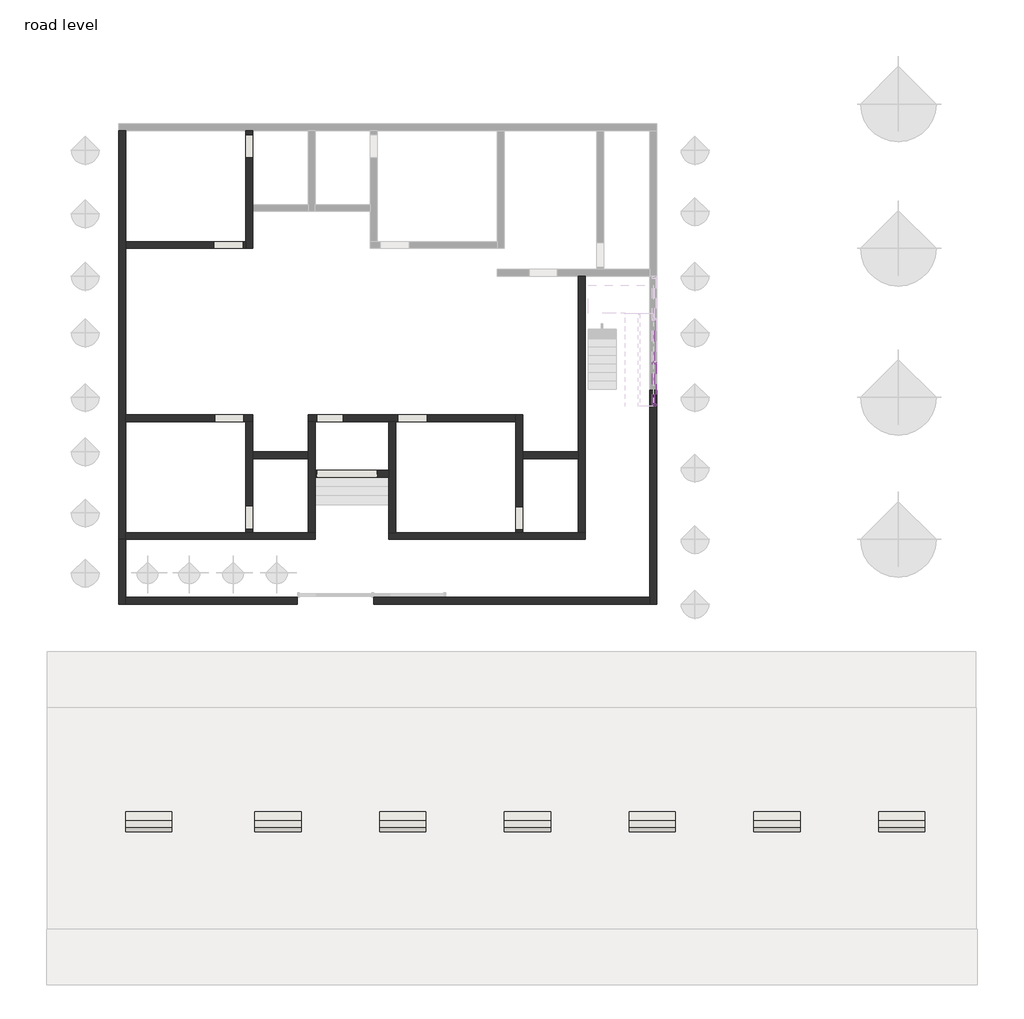
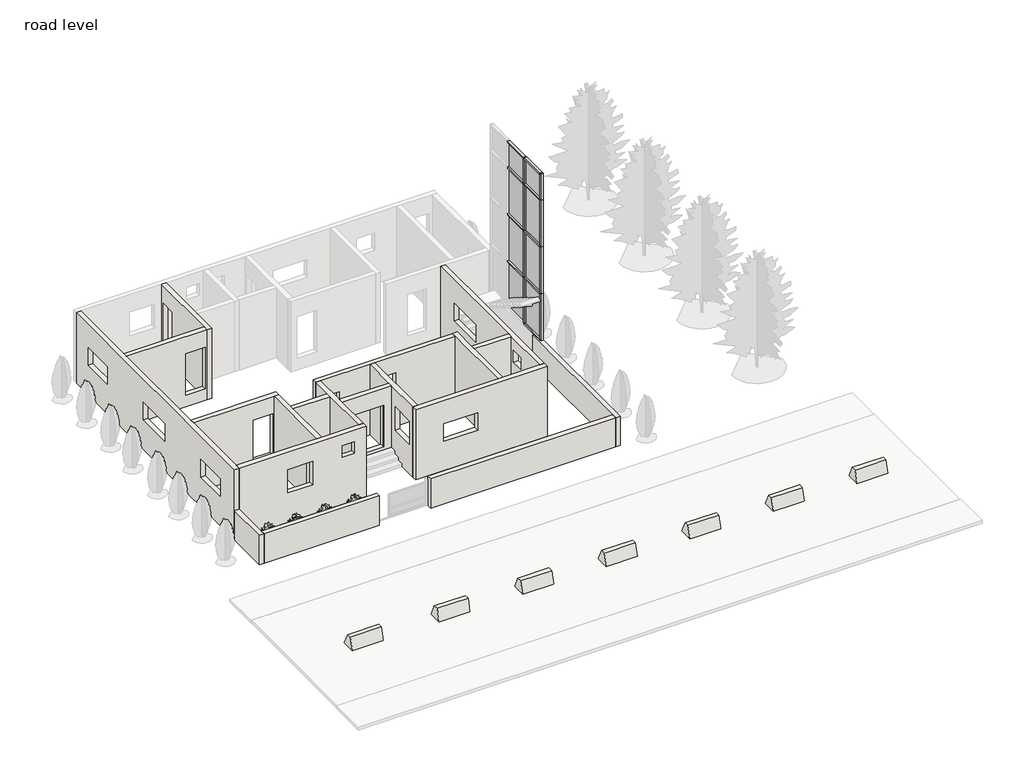
# One storey, part 1 of 2: 26 walls, 17 members, 8 plates.
"""IFC4 building model written with IfcOpenShell, lengths in millimetres."""

from ifc_helpers import new_model, si_unit, frame, origin, origin_with_axes, place, context, project, spatial, polyline, outline, extrude, faceted_brep, transform, mapped, element, save
from components import member_6e705821, member_22948727, member_0bf151aa, member_30211588, member_f0fea5a5, member_ee409385, member_824a4a8d, member_c6627131, system_panel_glazed_532211e4, system_panel_glazed_fddb435e, system_panel_glazed_e2c3efe7, system_panel_glazed_aadce453, system_panel_glazed_7e5d82eb, system_panel_glazed_fa23d52e

model = new_model("IFC4")

# Units and contexts
model_context = context("Model", 3, world=origin())
ifc_project = project(units=[si_unit("LENGTHUNIT", "METRE", prefix="MILLI")], contexts=[model_context])

# Site, building, storey
site = spatial("IfcSite", under=ifc_project)
building = spatial("IfcBuilding", under=site)
storey = spatial("IfcBuildingStorey", under=building, Name="road level", Elevation=0.0)

# Members
placement = place(None, origin())
member_shape = member_6e705821(model_context)
element("IfcMember", 1, ObjectType="Rectangular Mullion : 2.5\" x 5\" rectangular", at=placement, inside=storey, context=model_context, shape_type="MappedRepresentation", body=[
    mapped(member_shape, transform((9636.3894662, -2184.3339187, 10210.8), x_axis=(0.0, 0.0, 1.0), y_axis=(-1.0, 0.0, 0.0), z_axis=(0.0, -1.0, 0.0))),
])
member_2_shape = member_22948727(model_context)
element("IfcMember", 2, ObjectType="Rectangular Mullion : 2.5\" x 5\" rectangular", at=placement, inside=storey, context=model_context, shape_type="MappedRepresentation", body=[
    mapped(member_2_shape, transform((9636.3894662, -785.2172519, 10210.8), x_axis=(0.0, 0.0, 1.0), y_axis=(-1.0, 0.0, 0.0), z_axis=(0.0, -1.0, 0.0))),
])
element("IfcMember", 3, ObjectType="Rectangular Mullion : 2.5\" x 5\" rectangular", at=placement, inside=storey, context=model_context, shape_type="MappedRepresentation", body=[
    mapped(member_shape, transform((9636.3894662, -848.7172519, 1524.0), x_axis=(0.0, 0.0, -1.0), y_axis=(-1.0, 0.0, 0.0), z_axis=(0.0, 1.0, 0.0))),
])
member_3_shape = member_0bf151aa(model_context)
element("IfcMember", 4, ObjectType="Rectangular Mullion : 2.5\" x 5\" rectangular", at=placement, inside=storey, context=model_context, shape_type="MappedRepresentation", body=[
    mapped(member_3_shape, transform((9636.3894662, -2184.3339187, 3962.4), x_axis=(0.0, 0.0, 1.0), y_axis=(-1.0, 0.0, 0.0), z_axis=(0.0, -1.0, 0.0))),
])
element("IfcMember", 5, ObjectType="Rectangular Mullion : 2.5\" x 5\" rectangular", at=placement, inside=storey, context=model_context, shape_type="MappedRepresentation", body=[
    mapped(member_3_shape, transform((9636.3894662, -2184.3339187, 6400.8), x_axis=(0.0, 0.0, 1.0), y_axis=(-1.0, 0.0, 0.0), z_axis=(0.0, -1.0, 0.0))),
])
element("IfcMember", 6, ObjectType="Rectangular Mullion : 2.5\" x 5\" rectangular", at=placement, inside=storey, context=model_context, shape_type="MappedRepresentation", body=[
    mapped(member_3_shape, transform((9636.3894662, -2184.3339187, 8839.2), x_axis=(0.0, 0.0, 1.0), y_axis=(-1.0, 0.0, 0.0), z_axis=(0.0, -1.0, 0.0))),
])
member_4_shape = member_30211588(model_context)
element("IfcMember", 7, ObjectType="Rectangular Mullion : 2.5\" x 5\" rectangular", at=placement, inside=storey, context=model_context, shape_type="MappedRepresentation", body=[
    mapped(member_4_shape, transform((9636.3894662, -785.2172519, 3962.4), x_axis=(0.0, 0.0, 1.0), y_axis=(-1.0, 0.0, 0.0), z_axis=(0.0, -1.0, 0.0))),
])
element("IfcMember", 8, ObjectType="Rectangular Mullion : 2.5\" x 5\" rectangular", at=placement, inside=storey, context=model_context, shape_type="MappedRepresentation", body=[
    mapped(member_4_shape, transform((9636.3894662, -785.2172519, 6400.8), x_axis=(0.0, 0.0, 1.0), y_axis=(-1.0, 0.0, 0.0), z_axis=(0.0, -1.0, 0.0))),
])
element("IfcMember", 9, ObjectType="Rectangular Mullion : 2.5\" x 5\" rectangular", at=placement, inside=storey, context=model_context, shape_type="MappedRepresentation", body=[
    mapped(member_4_shape, transform((9636.3894662, -785.2172519, 8839.2), x_axis=(0.0, 0.0, 1.0), y_axis=(-1.0, 0.0, 0.0), z_axis=(0.0, -1.0, 0.0))),
])
member_5_shape = member_f0fea5a5(model_context)
element("IfcMember", 10, ObjectType="Rectangular Mullion : 2.5\" x 5\" rectangular", at=placement, inside=storey, context=model_context, shape_type="MappedRepresentation", body=[
    mapped(member_5_shape, transform((9636.3894662, -816.9672519, 1524.0), x_axis=(0.0, -1.0, 0.0), y_axis=(-1.0, 0.0, 0.0), z_axis=(0.0, 0.0, -1.0))),
])
element("IfcMember", 11, ObjectType="Rectangular Mullion : 2.5\" x 5\" rectangular", at=placement, inside=storey, context=model_context, shape_type="MappedRepresentation", body=[
    mapped(member_5_shape, transform((9636.3894662, -816.9672519, 3962.4), x_axis=(0.0, -1.0, 0.0), y_axis=(-1.0, 0.0, 0.0), z_axis=(0.0, 0.0, -1.0))),
])
element("IfcMember", 12, ObjectType="Rectangular Mullion : 2.5\" x 5\" rectangular", at=placement, inside=storey, context=model_context, shape_type="MappedRepresentation", body=[
    mapped(member_5_shape, transform((9636.3894662, -816.9672519, 6400.8), x_axis=(0.0, -1.0, 0.0), y_axis=(-1.0, 0.0, 0.0), z_axis=(0.0, 0.0, -1.0))),
])
member_6_shape = member_ee409385(model_context)
element("IfcMember", 13, ObjectType="Rectangular Mullion : 2.5\" x 5\" rectangular", at=placement, inside=storey, context=model_context, shape_type="MappedRepresentation", body=[
    mapped(member_6_shape, transform((9636.3894662, -2247.8339187, 1524.0), x_axis=(0.0, -1.0, 0.0), y_axis=(-1.0, 0.0, 0.0), z_axis=(0.0, 0.0, -1.0))),
])
element("IfcMember", 14, ObjectType="Rectangular Mullion : 2.5\" x 5\" rectangular", at=placement, inside=storey, context=model_context, shape_type="MappedRepresentation", body=[
    mapped(member_6_shape, transform((9636.3894662, -2247.8339187, 3962.4), x_axis=(0.0, -1.0, 0.0), y_axis=(-1.0, 0.0, 0.0), z_axis=(0.0, 0.0, -1.0))),
])
element("IfcMember", 15, ObjectType="Rectangular Mullion : 2.5\" x 5\" rectangular", at=placement, inside=storey, context=model_context, shape_type="MappedRepresentation", body=[
    mapped(member_6_shape, transform((9636.3894662, -2247.8339187, 6400.8), x_axis=(0.0, -1.0, 0.0), y_axis=(-1.0, 0.0, 0.0), z_axis=(0.0, 0.0, -1.0))),
])
member_7_shape = member_824a4a8d(model_context)
element("IfcMember", 16, ObjectType="Rectangular Mullion : 2.5\" x 5\" rectangular", at=placement, inside=storey, context=model_context, shape_type="MappedRepresentation", body=[
    mapped(member_7_shape, transform((9636.3894662, -816.9672519, 8839.2), x_axis=(0.0, -1.0, 0.0), y_axis=(-1.0, 0.0, 0.0), z_axis=(0.0, 0.0, -1.0))),
])
member_8_shape = member_c6627131(model_context)
element("IfcMember", 17, ObjectType="Rectangular Mullion : 2.5\" x 5\" rectangular", at=placement, inside=storey, context=model_context, shape_type="MappedRepresentation", body=[
    mapped(member_8_shape, transform((9636.3894662, -2247.8339187, 8839.2), x_axis=(0.0, -1.0, 0.0), y_axis=(-1.0, 0.0, 0.0), z_axis=(0.0, 0.0, -1.0))),
])

# Plates
system_panel_glazed_shape = system_panel_glazed_532211e4(model_context)
element("IfcPlate", 18, ObjectType="System Panel : Glazed", at=placement, inside=storey, context=model_context, shape_type="MappedRepresentation", body=[
    mapped(system_panel_glazed_shape, transform((9636.3894662, -1516.5255853, 1587.5), x_axis=(0.0, -1.0, 0.0), y_axis=(1.0, 0.0, 0.0), z_axis=(0.0, 0.0, 1.0))),
])
system_panel_glazed_2_shape = system_panel_glazed_fddb435e(model_context)
element("IfcPlate", 19, ObjectType="System Panel : Glazed", at=placement, inside=storey, context=model_context, shape_type="MappedRepresentation", body=[
    mapped(system_panel_glazed_2_shape, transform((9636.3894662, -101.5339187, 1587.5), x_axis=(0.0, -1.0, 0.0), y_axis=(1.0, 0.0, 0.0), z_axis=(0.0, 0.0, 1.0))),
])
system_panel_glazed_3_shape = system_panel_glazed_e2c3efe7(model_context)
element("IfcPlate", 20, ObjectType="System Panel : Glazed", at=placement, inside=storey, context=model_context, shape_type="MappedRepresentation", body=[
    mapped(system_panel_glazed_3_shape, transform((9636.3894662, -1516.5255853, 3994.15), x_axis=(0.0, -1.0, 0.0), y_axis=(1.0, 0.0, 0.0), z_axis=(0.0, 0.0, 1.0))),
])
element("IfcPlate", 21, ObjectType="System Panel : Glazed", at=placement, inside=storey, context=model_context, shape_type="MappedRepresentation", body=[
    mapped(system_panel_glazed_3_shape, transform((9636.3894662, -1516.5255853, 6432.55), x_axis=(0.0, -1.0, 0.0), y_axis=(1.0, 0.0, 0.0), z_axis=(0.0, 0.0, 1.0))),
])
system_panel_glazed_4_shape = system_panel_glazed_aadce453(model_context)
element("IfcPlate", 22, ObjectType="System Panel : Glazed", at=placement, inside=storey, context=model_context, shape_type="MappedRepresentation", body=[
    mapped(system_panel_glazed_4_shape, transform((9636.3894662, -101.5339187, 3994.15), x_axis=(0.0, -1.0, 0.0), y_axis=(1.0, 0.0, 0.0), z_axis=(0.0, 0.0, 1.0))),
])
element("IfcPlate", 23, ObjectType="System Panel : Glazed", at=placement, inside=storey, context=model_context, shape_type="MappedRepresentation", body=[
    mapped(system_panel_glazed_4_shape, transform((9636.3894662, -101.5339187, 6432.55), x_axis=(0.0, -1.0, 0.0), y_axis=(1.0, 0.0, 0.0), z_axis=(0.0, 0.0, 1.0))),
])
system_panel_glazed_5_shape = system_panel_glazed_7e5d82eb(model_context)
element("IfcPlate", 24, ObjectType="System Panel : Glazed", at=placement, inside=storey, context=model_context, shape_type="MappedRepresentation", body=[
    mapped(system_panel_glazed_5_shape, transform((9636.3894662, -1516.5255853, 8870.95), x_axis=(0.0, -1.0, 0.0), y_axis=(1.0, 0.0, 0.0), z_axis=(0.0, 0.0, 1.0))),
])
system_panel_glazed_6_shape = system_panel_glazed_fa23d52e(model_context)
element("IfcPlate", 25, ObjectType="System Panel : Glazed", at=placement, inside=storey, context=model_context, shape_type="MappedRepresentation", body=[
    mapped(system_panel_glazed_6_shape, transform((9636.3894662, -101.5339187, 8870.95), x_axis=(0.0, -1.0, 0.0), y_axis=(1.0, 0.0, 0.0), z_axis=(0.0, 0.0, 1.0))),
])

# Walls
element("IfcWall", 26, ObjectType="Generic - 9\"", at=placement, inside=storey, context=model_context, shape_type="Brep", body=[
    faceted_brep([(-8029.5739162, 6845.3660813, 0.0), (-8029.5739162, -6642.0339187, 0.0), (-8029.5739162, -6642.0339187, 1524.0), (-8029.5739162, -6642.0339187, 3657.6), (-8029.5739162, 6845.3660813, 3657.6), (-8029.5739162, 1143.0660813, 2438.4), (-8029.5739162, -685.7339187, 2438.4), (-8029.5739162, -685.7339187, 1524.0), (-8029.5739162, 1143.0660813, 1524.0), (-8029.5739162, 5842.0660813, 2438.4), (-8029.5739162, 4191.0660813, 2438.4), (-8029.5739162, 4191.0660813, 1524.0), (-8029.5739162, 5842.0660813, 1524.0), (-8029.5739162, -3759.1339187, 2438.4), (-8029.5739162, -5410.1339187, 2438.4), (-8029.5739162, -5410.1339187, 1524.0), (-8029.5739162, -3759.1339187, 1524.0), (-7800.9739162, 6845.3660813, 0.0), (-7800.9739162, 6845.3660813, 3657.6), (-7800.9739162, 3187.7660813, 3657.6), (-7800.9739162, 2959.1660813, 3657.6), (-7800.9739162, -2527.2339187, 3657.6), (-7800.9739162, -2755.8339187, 3657.6), (-7800.9739162, -6413.4339187, 3657.6), (-7800.9739162, -6642.0339187, 3657.6), (-7800.9739162, -6642.0339187, 1524.0), (-7800.9739162, -6642.0339187, 0.0), (-7800.9739162, -6413.4339187, 0.0), (-7800.9739162, -2755.8339187, 0.0), (-7800.9739162, -2527.2339187, 0.0), (-7800.9739162, 2959.1660813, 0.0), (-7800.9739162, 3187.7660813, 0.0), (-7800.9739162, 1143.0660813, 2438.4), (-7800.9739162, 1143.0660813, 1524.0), (-7800.9739162, -685.7339187, 1524.0), (-7800.9739162, -685.7339187, 2438.4), (-7800.9739162, 5842.0660813, 2438.4), (-7800.9739162, 5842.0660813, 1524.0), (-7800.9739162, 4191.0660813, 1524.0), (-7800.9739162, 4191.0660813, 2438.4), (-7800.9739162, -3759.1339187, 2438.4), (-7800.9739162, -3759.1339187, 1524.0), (-7800.9739162, -5410.1339187, 1524.0), (-7800.9739162, -5410.1339187, 2438.4)], [[[0, 1, 2, 3, 4], [5, 6, 7, 8], [9, 10, 11, 12], [13, 14, 15, 16]], [[17, 18, 19, 20, 21, 22, 23, 24, 25, 26, 27, 28, 29, 30, 31], [32, 33, 34, 35], [36, 37, 38, 39], [40, 41, 42, 43]], [[1, 0, 17, 31, 30, 29, 28, 27, 26]], [[0, 4, 18, 17]], [[33, 32, 5, 8]], [[34, 33, 8, 7]], [[35, 34, 7, 6]], [[32, 35, 6, 5]], [[37, 36, 9, 12]], [[38, 37, 12, 11]], [[39, 38, 11, 10]], [[36, 39, 10, 9]], [[41, 40, 13, 16]], [[42, 41, 16, 15]], [[43, 42, 15, 14]], [[40, 43, 14, 13]], [[1, 26, 25, 24, 3, 2]], [[4, 3, 24, 23, 22, 21, 20, 19, 18]]]),
])
element("IfcWall", 27, ObjectType="Generic - 9\"", at=placement, inside=storey, context=model_context, shape_type="Brep", body=[
    faceted_brep([(-3838.5739162, 6845.3660813, 0.0), (-3838.5739162, 3187.7660813, 0.0), (-3838.5739162, 2959.1660813, 0.0), (-3838.5739162, 2959.1660813, 3657.6), (-3838.5739162, 3187.7660813, 3657.6), (-3838.5739162, 6845.3660813, 3657.6), (-3838.5739162, 5943.6660813, 609.6), (-3838.5739162, 6705.6660813, 609.6), (-3838.5739162, 6705.6660813, 2743.2), (-3838.5739162, 5943.6660813, 2743.2), (-3609.9739162, 2959.1660813, 0.0), (-3609.9739162, 4178.3660813, 0.0), (-3609.9739162, 4406.9660813, 0.0), (-3609.9739162, 6845.3660813, 0.0), (-3609.9739162, 6845.3660813, 3657.6), (-3609.9739162, 4406.9660813, 3657.6), (-3609.9739162, 4178.3660813, 3657.6), (-3609.9739162, 2959.1660813, 3657.6), (-3609.9739162, 6705.6660813, 609.6), (-3609.9739162, 5943.6660813, 609.6), (-3609.9739162, 5943.6660813, 2743.2), (-3609.9739162, 6705.6660813, 2743.2)], [[[0, 1, 2, 3, 4, 5], [6, 7, 8, 9]], [[10, 11, 12, 13, 14, 15, 16, 17], [18, 19, 20, 21]], [[2, 1, 0, 13, 12, 11, 10]], [[0, 5, 14, 13]], [[3, 2, 10, 17]], [[6, 19, 18, 7]], [[7, 18, 21, 8]], [[19, 6, 9, 20]], [[20, 9, 8, 21]], [[5, 4, 3, 17, 16, 15, 14]]]),
])
element("IfcWall", 28, ObjectType="Generic - 9\"", at=placement, inside=storey, context=model_context, shape_type="SweptSolid", body=[
    extrude(outline(polyline([(0.0, -7800.9739162), (0.0, -3838.5739162), (3657.6, -3838.5739162), (3657.6, -7800.9739162), (0.0, -7800.9739162)]), holes=[polyline([(2768.6, -3927.4739162), (609.6, -3927.4739162), (609.6, -4892.6739162), (2768.6, -4892.6739162), (2768.6, -3927.4739162)])]), frame((0.0, 2959.1660813, 0.0), z_axis=(0.0, 1.0, 0.0), x_axis=(0.0, 0.0, 1.0)), (0.0, 0.0, 1.0), 228.6),
])
element("IfcWall", 29, ObjectType="Generic - 9\"", at=placement, inside=storey, context=model_context, shape_type="Brep", body=[
    faceted_brep([(-7800.9739162, -2755.8339187, 0.0), (-3838.5739162, -2755.8339187, 0.0), (-3609.9739162, -2755.8339187, 0.0), (-3609.9739162, -2755.8339187, 3657.6), (-3838.5739162, -2755.8339187, 3657.6), (-7800.9739162, -2755.8339187, 3657.6), (-3902.0739162, -2755.8339187, 2768.6), (-3902.0739162, -2755.8339187, 609.6), (-4867.2739162, -2755.8339187, 609.6), (-4867.2739162, -2755.8339187, 2768.6), (-3609.9739162, -2527.2339187, 0.0), (-7800.9739162, -2527.2339187, 0.0), (-7800.9739162, -2527.2339187, 3657.6), (-3609.9739162, -2527.2339187, 3657.6), (-3902.0739162, -2527.2339187, 609.6), (-3902.0739162, -2527.2339187, 2768.6), (-4867.2739162, -2527.2339187, 2768.6), (-4867.2739162, -2527.2339187, 609.6)], [[[0, 1, 2, 3, 4, 5], [6, 7, 8, 9]], [[10, 11, 12, 13], [14, 15, 16, 17]], [[2, 1, 0, 11, 10]], [[0, 5, 12, 11]], [[3, 2, 10, 13]], [[14, 7, 6, 15]], [[15, 6, 9, 16]], [[16, 9, 8, 17]], [[7, 14, 17, 8]], [[5, 4, 3, 13, 12]]]),
])
element("IfcWall", 30, ObjectType="Generic - 9\"", at=placement, inside=storey, context=model_context, shape_type="Brep", body=[
    faceted_brep([(-7800.9739162, -6642.0339187, 0.0), (-1552.5739162, -6642.0339187, 0.0), (-1552.5739162, -6642.0339187, 3657.6), (-1793.8739162, -6642.0339187, 3657.6), (-7800.9739162, -6642.0339187, 3657.6), (-5400.6739162, -6642.0339187, 1524.0), (-5400.6739162, -6642.0339187, 2743.2), (-4181.4739162, -6642.0339187, 2743.2), (-4181.4739162, -6642.0339187, 1524.0), (-2124.0739162, -6642.0339187, 3048.0), (-2124.0739162, -6642.0339187, 2438.4), (-2733.6739162, -6642.0339187, 2438.4), (-2733.6739162, -6642.0339187, 3048.0), (-1552.5739162, -6413.4339187, 0.0), (-1781.1739162, -6413.4339187, 0.0), (-3609.9739162, -6413.4339187, 0.0), (-3838.5739162, -6413.4339187, 0.0), (-7800.9739162, -6413.4339187, 0.0), (-7800.9739162, -6413.4339187, 3657.6), (-3838.5739162, -6413.4339187, 3657.6), (-3609.9739162, -6413.4339187, 3657.6), (-1781.1739162, -6413.4339187, 3657.6), (-1552.5739162, -6413.4339187, 3657.6), (-5400.6739162, -6413.4339187, 2743.2), (-5400.6739162, -6413.4339187, 1524.0), (-4181.4739162, -6413.4339187, 1524.0), (-4181.4739162, -6413.4339187, 2743.2), (-2124.0739162, -6413.4339187, 2438.4), (-2124.0739162, -6413.4339187, 3048.0), (-2733.6739162, -6413.4339187, 3048.0), (-2733.6739162, -6413.4339187, 2438.4)], [[[0, 1, 2, 3, 4], [5, 6, 7, 8], [9, 10, 11, 12]], [[13, 14, 15, 16, 17, 18, 19, 20, 21, 22], [23, 24, 25, 26], [27, 28, 29, 30]], [[1, 0, 17, 16, 15, 14, 13]], [[2, 1, 13, 22]], [[23, 6, 5, 24]], [[24, 5, 8, 25]], [[25, 8, 7, 26]], [[6, 23, 26, 7]], [[10, 9, 28, 27]], [[11, 10, 27, 30]], [[12, 11, 30, 29]], [[9, 12, 29, 28]], [[4, 18, 17, 0]], [[22, 21, 20, 19, 18, 4, 3, 2]]]),
])
element("IfcWall", 31, ObjectType="Generic - 9\"", at=placement, inside=storey, context=model_context, shape_type="Brep", body=[
    faceted_brep([(-3609.9739162, -6413.4339187, 0.0), (-3609.9739162, -3975.0339187, 0.0), (-3609.9739162, -3746.4339187, 0.0), (-3609.9739162, -2755.8339187, 0.0), (-3609.9739162, -2755.8339187, 3657.6), (-3609.9739162, -3746.4339187, 3657.6), (-3609.9739162, -3975.0339187, 3657.6), (-3609.9739162, -6413.4339187, 3657.6), (-3609.9739162, -5537.1339187, 609.6), (-3609.9739162, -6299.1339187, 609.6), (-3609.9739162, -6299.1339187, 2743.2), (-3609.9739162, -5537.1339187, 2743.2), (-3838.5739162, -2755.8339187, 0.0), (-3838.5739162, -6413.4339187, 0.0), (-3838.5739162, -6413.4339187, 3657.6), (-3838.5739162, -2755.8339187, 3657.6), (-3838.5739162, -6299.1339187, 609.6), (-3838.5739162, -5537.1339187, 609.6), (-3838.5739162, -5537.1339187, 2743.2), (-3838.5739162, -6299.1339187, 2743.2)], [[[0, 1, 2, 3, 4, 5, 6, 7], [8, 9, 10, 11]], [[12, 13, 14, 15], [16, 17, 18, 19]], [[3, 2, 1, 0, 13, 12]], [[0, 7, 14, 13]], [[4, 3, 12, 15]], [[8, 17, 16, 9]], [[9, 16, 19, 10]], [[17, 8, 11, 18]], [[18, 11, 10, 19]], [[7, 6, 5, 4, 15, 14]]]),
])
element("IfcWall", 32, ObjectType="Generic - 9\"", at=placement, inside=storey, context=model_context, shape_type="Brep", body=[
    faceted_brep([(-1781.1739162, -2755.8339187, 0.0), (-1781.1739162, -3746.4339187, 0.0), (-1781.1739162, -3975.0339187, 0.0), (-1781.1739162, -6413.4339187, 0.0), (-1781.1739162, -6413.4339187, 3657.6), (-1781.1739162, -3975.0339187, 3657.6), (-1781.1739162, -3746.4339187, 3657.6), (-1781.1739162, -2755.8339187, 3657.6), (-1552.5739162, -2755.8339187, 0.0), (-1552.5739162, -2755.8339187, 3657.6), (-1552.5739162, -4356.0339187, 3657.6), (-1552.5739162, -4584.6339187, 3657.6), (-1552.5739162, -6413.4339187, 3657.6), (-1552.5739162, -6413.4339187, 0.0), (-1552.5739162, -4584.6339187, 0.0), (-1552.5739162, -4356.0339187, 0.0)], [[[0, 1, 2, 3, 4, 5, 6, 7]], [[8, 9, 10, 11, 12, 13, 14, 15]], [[3, 2, 1, 0, 8, 15, 14, 13]], [[0, 7, 9, 8]], [[4, 3, 13, 12]], [[7, 6, 5, 4, 12, 11, 10, 9]]]),
])
element("IfcWall", 33, ObjectType="Generic - 9\"", at=placement, inside=storey, context=model_context, shape_type="SweptSolid", body=[
    extrude(outline(polyline([(-3609.9739162, -3746.4339187), (-1781.1739162, -3746.4339187), (-1781.1739162, -3975.0339187), (-3609.9739162, -3975.0339187), (-3609.9739162, -3746.4339187)])), origin_with_axes(), (0.0, 0.0, 1.0), 3657.6),
])
element("IfcWall", 34, ObjectType="Generic - 9\"", at=placement, inside=storey, context=model_context, shape_type="Brep", body=[
    faceted_brep([(1114.4260838, -6413.4339187, 0.0), (1114.4260838, -2755.8339187, 0.0), (1114.4260838, -2755.8339187, 3657.6), (1114.4260838, -6413.4339187, 3657.6), (1114.4260838, -4889.4339187, 2743.2), (1114.4260838, -4889.4339187, 1524.0), (1114.4260838, -6108.6339187, 1524.0), (1114.4260838, -6108.6339187, 2743.2), (885.8260838, -2755.8339187, 0.0), (885.8260838, -4356.0339187, 0.0), (885.8260838, -4584.6339187, 0.0), (885.8260838, -6413.4339187, 0.0), (885.8260838, -6413.4339187, 3657.6), (885.8260838, -4584.6339187, 3657.6), (885.8260838, -4356.0339187, 3657.6), (885.8260838, -2755.8339187, 3657.6), (885.8260838, -4889.4339187, 1524.0), (885.8260838, -4889.4339187, 2743.2), (885.8260838, -6108.6339187, 2743.2), (885.8260838, -6108.6339187, 1524.0)], [[[0, 1, 2, 3], [4, 5, 6, 7]], [[8, 9, 10, 11, 12, 13, 14, 15], [16, 17, 18, 19]], [[1, 0, 11, 10, 9, 8]], [[2, 1, 8, 15]], [[0, 3, 12, 11]], [[4, 17, 16, 5]], [[5, 16, 19, 6]], [[6, 19, 18, 7]], [[17, 4, 7, 18]], [[3, 2, 15, 14, 13, 12]]]),
])
element("IfcWall", 35, ObjectType="Generic - 9\"", at=placement, inside=storey, context=model_context, shape_type="Brep", body=[
    faceted_brep([(5076.8260838, -2527.2339187, 0.0), (-1781.1739162, -2527.2339187, 0.0), (-1781.1739162, -2527.2339187, 3657.6), (5076.8260838, -2527.2339187, 3657.6), (1177.9260838, -2527.2339187, 2768.6), (1177.9260838, -2527.2339187, 609.6), (2143.1260838, -2527.2339187, 609.6), (2143.1260838, -2527.2339187, 2768.6), (-1489.0739162, -2527.2339187, 2768.6), (-1489.0739162, -2527.2339187, 609.6), (-625.4739162, -2527.2339187, 609.6), (-625.4739162, -2527.2339187, 2768.6), (-1781.1739162, -2755.8339187, 0.0), (-1552.5739162, -2755.8339187, 0.0), (885.8260838, -2755.8339187, 0.0), (1114.4260838, -2755.8339187, 0.0), (5076.8260838, -2755.8339187, 0.0), (5076.8260838, -2755.8339187, 3657.6), (1114.4260838, -2755.8339187, 3657.6), (885.8260838, -2755.8339187, 3657.6), (-1552.5739162, -2755.8339187, 3657.6), (-1781.1739162, -2755.8339187, 3657.6), (1177.9260838, -2755.8339187, 609.6), (1177.9260838, -2755.8339187, 2768.6), (2143.1260838, -2755.8339187, 2768.6), (2143.1260838, -2755.8339187, 609.6), (-1489.0739162, -2755.8339187, 609.6), (-1489.0739162, -2755.8339187, 2768.6), (-625.4739162, -2755.8339187, 2768.6), (-625.4739162, -2755.8339187, 609.6)], [[[0, 1, 2, 3], [4, 5, 6, 7], [8, 9, 10, 11]], [[12, 13, 14, 15, 16, 17, 18, 19, 20, 21], [22, 23, 24, 25], [26, 27, 28, 29]], [[1, 0, 16, 15, 14, 13, 12]], [[2, 1, 12, 21]], [[0, 3, 17, 16]], [[22, 5, 4, 23]], [[23, 4, 7, 24]], [[24, 7, 6, 25]], [[5, 22, 25, 6]], [[26, 9, 8, 27]], [[27, 8, 11, 28]], [[10, 29, 28, 11]], [[9, 26, 29, 10]], [[3, 2, 21, 20, 19, 18, 17]]]),
])
element("IfcWall", 36, ObjectType="Generic - 9\"", at=placement, inside=storey, context=model_context, shape_type="Brep", body=[
    faceted_brep([(5305.4260838, -6413.4339187, 0.0), (5305.4260838, -3975.0339187, 0.0), (5305.4260838, -3746.4339187, 0.0), (5305.4260838, -2527.2339187, 0.0), (5305.4260838, -2527.2339187, 3657.6), (5305.4260838, -3746.4339187, 3657.6), (5305.4260838, -3975.0339187, 3657.6), (5305.4260838, -6413.4339187, 3657.6), (5305.4260838, -5562.5339187, 609.6), (5305.4260838, -6324.5339187, 609.6), (5305.4260838, -6324.5339187, 2743.2), (5305.4260838, -5562.5339187, 2743.2), (5076.8260838, -2527.2339187, 0.0), (5076.8260838, -2755.8339187, 0.0), (5076.8260838, -6413.4339187, 0.0), (5076.8260838, -6413.4339187, 3657.6), (5076.8260838, -2755.8339187, 3657.6), (5076.8260838, -2527.2339187, 3657.6), (5076.8260838, -6324.5339187, 609.6), (5076.8260838, -5562.5339187, 609.6), (5076.8260838, -5562.5339187, 2743.2), (5076.8260838, -6324.5339187, 2743.2)], [[[0, 1, 2, 3, 4, 5, 6, 7], [8, 9, 10, 11]], [[12, 13, 14, 15, 16, 17], [18, 19, 20, 21]], [[3, 2, 1, 0, 14, 13, 12]], [[0, 7, 15, 14]], [[4, 3, 12, 17]], [[8, 19, 18, 9]], [[9, 18, 21, 10]], [[19, 8, 11, 20]], [[20, 11, 10, 21]], [[7, 6, 5, 4, 17, 16, 15]]]),
])
element("IfcWall", 37, ObjectType="Generic - 9\"", at=placement, inside=storey, context=model_context, shape_type="Brep", body=[
    faceted_brep([(7362.8260838, -6413.4339187, 0.0), (7362.8260838, 2044.7660813, 0.0), (7362.8260838, 2044.7660813, 3657.6), (7362.8260838, -1689.0339187, 3657.6), (7362.8260838, -6413.4339187, 3657.6), (7362.8260838, -939.7339187, 1524.0), (7362.8260838, -939.7339187, 2438.4), (7362.8260838, 889.0660813, 2438.4), (7362.8260838, 889.0660813, 1524.0), (7362.8260838, -4165.5339187, 3048.0), (7362.8260838, -4165.5339187, 2438.4), (7362.8260838, -4775.1339187, 2438.4), (7362.8260838, -4775.1339187, 3048.0), (7134.2260838, 2044.7660813, 0.0), (7134.2260838, -3746.4339187, 0.0), (7134.2260838, -3975.0339187, 0.0), (7134.2260838, -6413.4339187, 0.0), (7134.2260838, -6413.4339187, 3657.6), (7134.2260838, -3975.0339187, 3657.6), (7134.2260838, -3746.4339187, 3657.6), (7134.2260838, 2044.7660813, 3657.6), (7134.2260838, -939.7339187, 2438.4), (7134.2260838, -939.7339187, 1524.0), (7134.2260838, 889.0660813, 1524.0), (7134.2260838, 889.0660813, 2438.4), (7134.2260838, -4165.5339187, 2438.4), (7134.2260838, -4165.5339187, 3048.0), (7134.2260838, -4775.1339187, 3048.0), (7134.2260838, -4775.1339187, 2438.4)], [[[0, 1, 2, 3, 4], [5, 6, 7, 8], [9, 10, 11, 12]], [[13, 14, 15, 16, 17, 18, 19, 20], [21, 22, 23, 24], [25, 26, 27, 28]], [[1, 0, 16, 15, 14, 13]], [[2, 1, 13, 20]], [[0, 4, 17, 16]], [[21, 6, 5, 22]], [[22, 5, 8, 23]], [[23, 8, 7, 24]], [[6, 21, 24, 7]], [[10, 9, 26, 25]], [[11, 10, 25, 28]], [[12, 11, 28, 27]], [[9, 12, 27, 26]], [[20, 19, 18, 17, 4, 3, 2]]]),
])
element("IfcWall", 38, ObjectType="Generic - 9\"", at=placement, inside=storey, context=model_context, shape_type="SweptSolid", body=[
    extrude(outline(polyline([(5305.4260838, -3746.4339187), (7134.2260838, -3746.4339187), (7134.2260838, -3975.0339187), (5305.4260838, -3975.0339187), (5305.4260838, -3746.4339187)])), origin_with_axes(), (0.0, 0.0, 1.0), 3657.6),
])
element("IfcWall", 39, ObjectType="Generic - 9\"", at=placement, inside=storey, context=model_context, shape_type="Brep", body=[
    faceted_brep([(885.8260838, -6642.0339187, 0.0), (7362.8260838, -6642.0339187, 0.0), (7362.8260838, -6642.0339187, 3657.6), (885.8260838, -6642.0339187, 3657.6), (2282.8260838, -6642.0339187, 1524.0), (2282.8260838, -6642.0339187, 2438.4), (3933.8260838, -6642.0339187, 2438.4), (3933.8260838, -6642.0339187, 1524.0), (7362.8260838, -6413.4339187, 0.0), (7134.2260838, -6413.4339187, 0.0), (5305.4260838, -6413.4339187, 0.0), (5076.8260838, -6413.4339187, 0.0), (1114.4260838, -6413.4339187, 0.0), (885.8260838, -6413.4339187, 0.0), (885.8260838, -6413.4339187, 3657.6), (1114.4260838, -6413.4339187, 3657.6), (5076.8260838, -6413.4339187, 3657.6), (5305.4260838, -6413.4339187, 3657.6), (7134.2260838, -6413.4339187, 3657.6), (7362.8260838, -6413.4339187, 3657.6), (2282.8260838, -6413.4339187, 2438.4), (2282.8260838, -6413.4339187, 1524.0), (3933.8260838, -6413.4339187, 1524.0), (3933.8260838, -6413.4339187, 2438.4)], [[[0, 1, 2, 3], [4, 5, 6, 7]], [[8, 9, 10, 11, 12, 13, 14, 15, 16, 17, 18, 19], [20, 21, 22, 23]], [[1, 0, 13, 12, 11, 10, 9, 8]], [[2, 1, 8, 19]], [[0, 3, 14, 13]], [[20, 5, 4, 21]], [[21, 4, 7, 22]], [[22, 7, 6, 23]], [[5, 20, 23, 6]], [[3, 2, 19, 18, 17, 16, 15, 14]]]),
])
element("IfcWall", 40, ObjectType="Generic - 9\"", at=placement, inside=storey, context=model_context, shape_type="Brep", body=[
    faceted_brep([(-1552.5739162, -4584.6339187, 0.0), (885.8260838, -4584.6339187, 0.0), (885.8260838, -4584.6339187, 3657.6), (-1552.5739162, -4584.6339187, 3657.6), (-1498.4739162, -4584.6339187, 2779.1), (501.5260838, -4584.6339187, 2779.1), (501.5260838, -4584.6339187, 609.6), (-1498.4739162, -4584.6339187, 609.6), (885.8260838, -4356.0339187, 0.0), (-1552.5739162, -4356.0339187, 0.0), (-1552.5739162, -4356.0339187, 3657.6), (885.8260838, -4356.0339187, 3657.6), (501.5260838, -4356.0339187, 2779.1), (-1498.4739162, -4356.0339187, 2779.1), (-1498.4739162, -4356.0339187, 609.6), (501.5260838, -4356.0339187, 609.6), (-1498.4739162, -4564.6339187, 2779.1), (501.5260838, -4564.6339187, 2779.1), (501.5260838, -4494.6339187, 2779.1), (-1498.4739162, -4494.6339187, 2779.1), (-1498.4739162, -4494.6339187, 609.6), (-1513.4739162, -4494.6339187, 609.6), (-1513.4739162, -4564.6339187, 609.6), (-1498.4739162, -4564.6339187, 609.6), (501.5260838, -4564.6339187, 609.6), (516.5260838, -4564.6339187, 609.6), (516.5260838, -4494.6339187, 609.6), (501.5260838, -4494.6339187, 609.6), (516.5260838, -4494.6339187, 2794.1), (-1513.4739162, -4494.6339187, 2794.1), (516.5260838, -4564.6339187, 2794.1), (-1513.4739162, -4564.6339187, 2794.1)], [[[0, 1, 2, 3], [4, 5, 6, 7]], [[8, 9, 10, 11], [12, 13, 14, 15]], [[1, 0, 9, 8]], [[0, 3, 10, 9]], [[2, 1, 8, 11]], [[16, 17, 5, 4]], [[18, 19, 13, 12]], [[20, 21, 22, 23, 7, 6, 24, 25, 26, 27, 15, 14]], [[19, 20, 14, 13]], [[27, 18, 12, 15]], [[19, 18, 27, 26, 28, 29, 21, 20]], [[26, 25, 30, 28]], [[17, 16, 23, 22, 31, 30, 25, 24]], [[17, 24, 6, 5]], [[23, 16, 4, 7]], [[22, 21, 29, 31]], [[29, 28, 30, 31]], [[3, 2, 11, 10]]]),
])
element("IfcWall", 41, ObjectType="Generic - 9\"", at=placement, inside=storey, context=model_context, shape_type="Brep", body=[
    faceted_brep([(-8029.5739162, -6642.0339187, 0.0), (-8029.5739162, -8775.0319901, 0.0), (-8029.5739162, -8775.0319901, 1524.0), (-8029.5739162, -6642.0339187, 1524.0), (-7800.9739162, -6642.0339187, 0.0), (-7800.9739162, -6642.0339187, 1524.0), (-7800.9739162, -8546.4319901, 1524.0), (-7800.9739162, -8775.0319901, 1524.0), (-7800.9739162, -8775.0319901, 0.0), (-7800.9739162, -8546.4319901, 0.0)], [[[0, 1, 2, 3]], [[4, 5, 6, 7, 8, 9]], [[1, 0, 4, 9, 8]], [[3, 2, 7, 6, 5]], [[0, 3, 5, 4]], [[2, 1, 8, 7]]]),
])
element("IfcWall", 42, ObjectType="Generic - 9\"", at=placement, inside=storey, context=model_context, shape_type="Brep", body=[
    faceted_brep([(9725.0260838, -8775.0319901, 0.0), (9725.0260838, -1714.4339187, 0.0), (9725.0260838, -1714.4339187, 1524.0), (9725.0260838, -8775.0319901, 1524.0), (9496.4260838, -8775.0319901, 0.0), (9496.4260838, -8775.0319901, 1524.0), (9496.4260838, -8546.4319901, 1524.0), (9496.4260838, -1714.4339187, 1524.0), (9496.4260838, -1714.4339187, 0.0), (9496.4260838, -8546.4319901, 0.0), (9496.6894662, -1714.4339187, 0.0), (9496.6894662, -1714.4339187, 1524.0)], [[[0, 1, 2, 3]], [[4, 5, 6, 7, 8, 9]], [[1, 0, 4, 9, 8, 10]], [[2, 1, 10, 8, 7, 11]], [[3, 2, 11, 7, 6, 5]], [[0, 3, 5, 4]]]),
])
element("IfcWall", 43, ObjectType="Generic - 9\"", at=placement, inside=storey, context=model_context, shape_type="SweptSolid", body=[
    extrude(outline(polyline([(-2130.4239162, -8775.0319901), (-7800.9739162, -8775.0319901), (-7800.9739162, -8546.4319901), (-2130.4239162, -8546.4319901), (-2130.4239162, -8775.0319901)])), origin_with_axes(), (0.0, 0.0, 1.0), 1524.0),
])
element("IfcWall", 44, ObjectType="Generic - 9\"", at=placement, inside=storey, context=model_context, shape_type="SweptSolid", body=[
    extrude(outline(polyline([(390.5260838, -8546.4319901), (9496.4260838, -8546.4319901), (9496.4260838, -8775.0319901), (390.5260838, -8775.0319901), (390.5260838, -8546.4319901)])), origin_with_axes(), (0.0, 0.0, 1.0), 1524.0),
])
element("IfcWall", 45, ObjectType="Generic - 9\"", at=placement, inside=storey, context=model_context, shape_type="SweptSolid", body=[
    extrude(outline(polyline([(-15615.4708417, 0.0), (-16291.6738178, 0.0), (-16128.3319901, 609.6), (-15899.7319901, 609.6), (-15615.4708417, 0.0)])), frame((-7800.9739162, 0.0, 0.0), z_axis=(1.0, 0.0, 0.0), x_axis=(0.0, 1.0, 0.0)), (0.0, 0.0, 1.0), 1524.0),
])
element("IfcWall", 46, ObjectType="Generic - 9\"", at=placement, inside=storey, context=model_context, shape_type="SweptSolid", body=[
    extrude(outline(polyline([(-15615.4708417, 0.0), (-16291.6738178, 0.0), (-16128.3319901, 609.6), (-15899.7319901, 609.6), (-15615.4708417, 0.0)])), frame((-3533.7739162, 0.0, 0.0), z_axis=(1.0, 0.0, 0.0), x_axis=(0.0, 1.0, 0.0)), (0.0, 0.0, 1.0), 1524.0),
])
element("IfcWall", 47, ObjectType="Generic - 9\"", at=placement, inside=storey, context=model_context, shape_type="SweptSolid", body=[
    extrude(outline(polyline([(-15615.4708417, 0.0), (-16291.6738178, 0.0), (-16128.3319901, 609.6), (-15899.7319901, 609.6), (-15615.4708417, 0.0)])), frame((581.0260838, 0.0, 0.0), z_axis=(1.0, 0.0, 0.0), x_axis=(0.0, 1.0, 0.0)), (0.0, 0.0, 1.0), 1524.0),
])
element("IfcWall", 48, ObjectType="Generic - 9\"", at=placement, inside=storey, context=model_context, shape_type="SweptSolid", body=[
    extrude(outline(polyline([(-15615.4708417, 0.0), (-16291.6738178, 0.0), (-16128.3319901, 609.6), (-15899.7319901, 609.6), (-15615.4708417, 0.0)])), frame((4695.8260838, 0.0, 0.0), z_axis=(1.0, 0.0, 0.0), x_axis=(0.0, 1.0, 0.0)), (0.0, 0.0, 1.0), 1524.0),
])
element("IfcWall", 49, ObjectType="Generic - 9\"", at=placement, inside=storey, context=model_context, shape_type="SweptSolid", body=[
    extrude(outline(polyline([(-15615.4708417, 0.0), (-16291.6738178, 0.0), (-16128.3319901, 609.6), (-15899.7319901, 609.6), (-15615.4708417, 0.0)])), frame((8810.6260838, 0.0, 0.0), z_axis=(1.0, 0.0, 0.0), x_axis=(0.0, 1.0, 0.0)), (0.0, 0.0, 1.0), 1524.0),
])
element("IfcWall", 50, ObjectType="Generic - 9\"", at=placement, inside=storey, context=model_context, shape_type="SweptSolid", body=[
    extrude(outline(polyline([(-15615.4708417, 0.0), (-16291.6738178, 0.0), (-16128.3319901, 609.6), (-15899.7319901, 609.6), (-15615.4708417, 0.0)])), frame((12925.4260838, 0.0, 0.0), z_axis=(1.0, 0.0, 0.0), x_axis=(0.0, 1.0, 0.0)), (0.0, 0.0, 1.0), 1524.0),
])
element("IfcWall", 51, ObjectType="Generic - 9\"", at=placement, inside=storey, context=model_context, shape_type="SweptSolid", body=[
    extrude(outline(polyline([(-15615.4708417, 0.0), (-16291.6738178, 0.0), (-16128.3319901, 609.6), (-15899.7319901, 609.6), (-15615.4708417, 0.0)])), frame((17040.2260838, 0.0, 0.0), z_axis=(1.0, 0.0, 0.0), x_axis=(0.0, 1.0, 0.0)), (0.0, 0.0, 1.0), 1524.0),
])

save(model, "model.ifc")

# Revit data of these elements
# Type "Rectangular Mullion : 2.5\" x 5\" rectangular"
#   built-in parameter 1007304 = 0.416667 (stored number, unit not read)
#   built-in parameter 1007301 = 0.104167 (stored number, unit not read)
#   built-in parameter 1007300 = 0.104167 (stored number, unit not read)
# Type "System Panel : Glazed"
#   Construction Type Id = "GSP4R"
#   Analytic Construction = "1/8 in Pilkington single glazing"
#   Visual Light Transmittance = 0.9
#   Solar Heat Gain Coefficient = 0.86
#   Heat Transfer Coefficient (U) = 1.18115 BTU/(h·ft²·°F)
#   Define Thermal Properties by = 1
# Type "Generic - 9\""
#   Assembly Code = "B2010"
#   Layers, outside or top first: 0' - 9" no material (function 1)
# Elements 1, 2, 3, 4, 5, 6, 7, 8, 9, 10, 11, 12, 13, 14, 15, 16, 17 (IfcMember, "Rectangular Mullion : 2.5\" x 5\" rectangular")
#   Phase Created = New Construction
#   Materials on its faces: "Aluminum"
# Elements 18, 19, 20, 21, 22, 23, 24, 25 (IfcPlate, "System Panel : Glazed")
#   Phase Created = New Construction
#   Materials on its faces: "Glass"
# Elements 26, 27, 28, 29, 30, 31, 32, 33, 34, 35, 36, 37, 38, 39, 40 (IfcWall, "Generic - 9\"")
#   Top Offset = 0' - 0"
#   Base Offset = 0' - 0"
#   wall height = 12' - 0"
#   Phase Created = New Construction
#   Base Constraint = road level
#   Top Constraint = 1st floor
#   Materials on its faces: "Default Wall"
# Elements 41, 42, 43, 44 (IfcWall, "Generic - 9\"")
#   Top Offset = 0' - 0"
#   Base Offset = 0' - 0"
#   Unconnected Height = 5' - 0"
#   wall height = 5' - 0"
#   Phase Created = New Construction
#   Base Constraint = road level
#   Materials on its faces: "Default Wall"
# Elements 45, 46, 47, 48, 49, 50, 51 (IfcWall, "Generic - 9\"")
#   Top Offset = 0' - 0"
#   Base Offset = 0' - 0"
#   wall height = 2' - 0"
#   Phase Created = New Construction
#   Base Constraint = road level
#   Top Constraint = ground level
#   Materials on its faces: "Default Wall"
# Materials
#   "Aluminum": class "Metal", colour RGB 247 247 247, transparency 0, Description = "Aluminum 6061", Cost = 0
#   "Glass": class "Glass", colour RGB 0 128 192, transparency 0.75, Description = "Soda Lime Glass", Cost = 0
#   "Default Wall": colour RGB 128 128 128, transparency 0, Cost = 0
